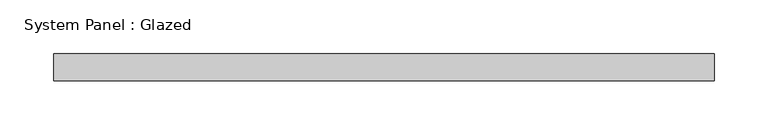
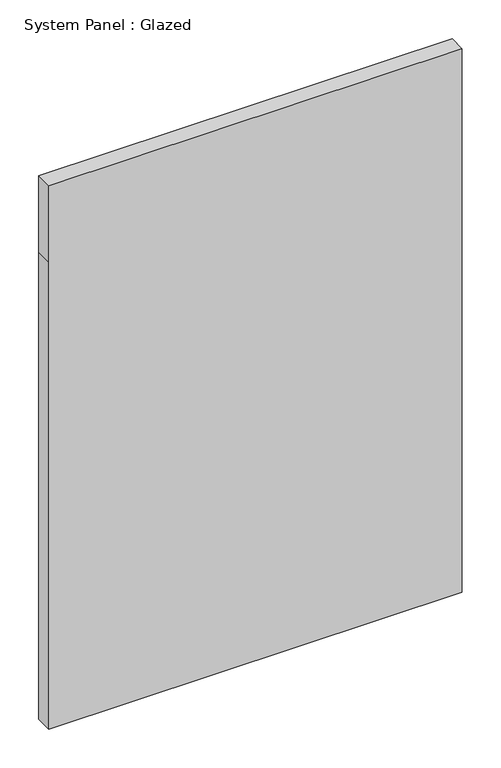
"""IFC4 building model written with IfcOpenShell, lengths in millimetres: plate geometry, System Panel : Glazed."""

from ifc_helpers import new_model, si_unit, frame, origin, place, context, project, spatial, polyline, outline, extrude, source, transform, mapped, element, save


def system_panel_glazed_52878f21(model_context):
    return source(origin(), model_context, "Body", "SweptSolid", [
        extrude(outline(polyline([(0.0, -307.975), (0.0, 307.975), (735.0443895, 307.975), (855.6943895, 307.975), (855.6943895, -307.975), (735.0443895, -307.975), (0.0, -307.975)])), frame((0.0, 19.05, 0.0), z_axis=(0.0, 1.0, 0.0), x_axis=(0.0, 0.0, 1.0)), (0.0, 0.0, 1.0), 25.4),
    ])


if __name__ == "__main__":
    model = new_model("IFC4")
    model_context = context("Model", 3, world=origin())
    ifc_project = project(units=[si_unit("LENGTHUNIT", "METRE", prefix="MILLI")], contexts=[model_context])
    site = spatial("IfcSite", under=ifc_project)
    building = spatial("IfcBuilding", under=site)
    placement = place(None, origin())
    system_panel_glazed_shape = system_panel_glazed_52878f21(model_context)
    element("IfcPlate", 1, ObjectType="System Panel : Glazed", at=placement, inside=building, context=model_context, shape_type="MappedRepresentation", body=[
        mapped(system_panel_glazed_shape, transform((0.0, 0.0, 0.0), x_axis=(1.0, 0.0, 0.0), y_axis=(0.0, 1.0, 0.0), z_axis=(0.0, 0.0, 1.0))),
    ])
    save(model, "model.ifc")

# Revit data of these elements
# Type "System Panel : Glazed"
#   Construction Type Id = "GSP4R"
#   Analytic Construction = "1/8 in Pilkington single glazing"
#   Visual Light Transmittance = 0.9
#   Solar Heat Gain Coefficient = 0.86
#   Heat Transfer Coefficient (U) = 1.18115 BTU/(h·ft²·°F)
#   Define Thermal Properties by = 1
# Element 1 (IfcPlate, "System Panel : Glazed")
#   Materials on its faces: "Glass"
# Materials
#   "Glass": class "Glass", colour RGB 0 128 192, transparency 0.75, Description = "Soda Lime Glass", Cost = 0
